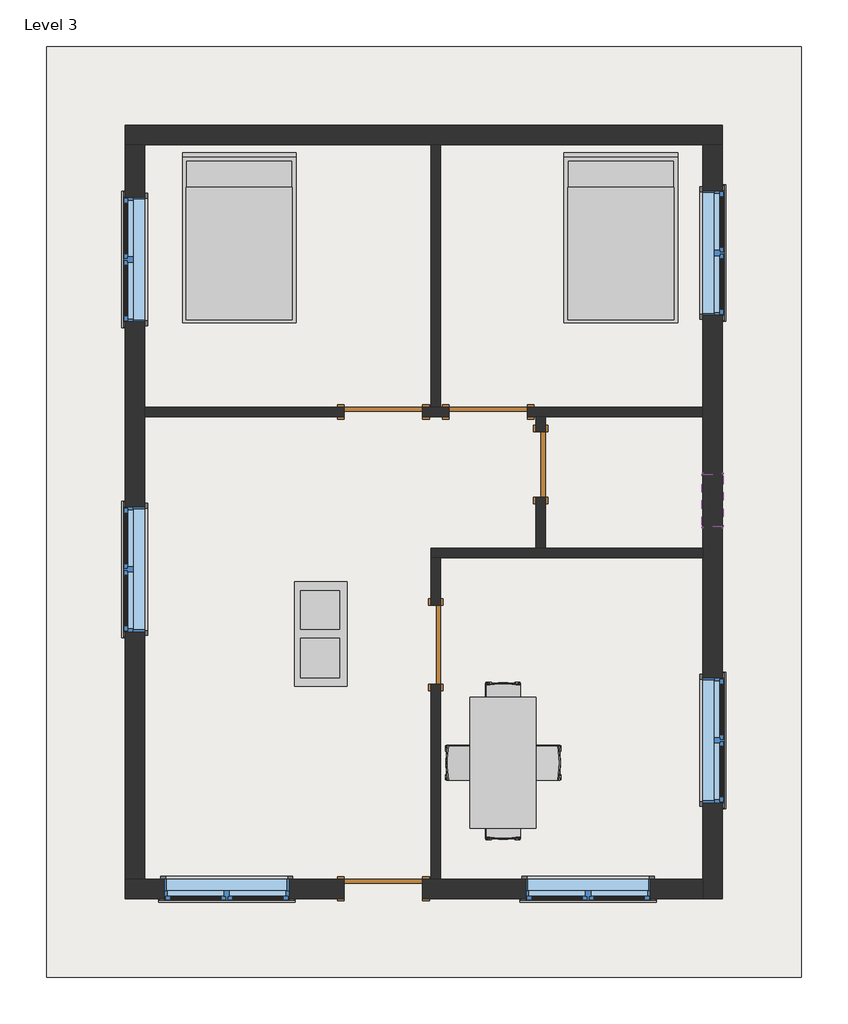
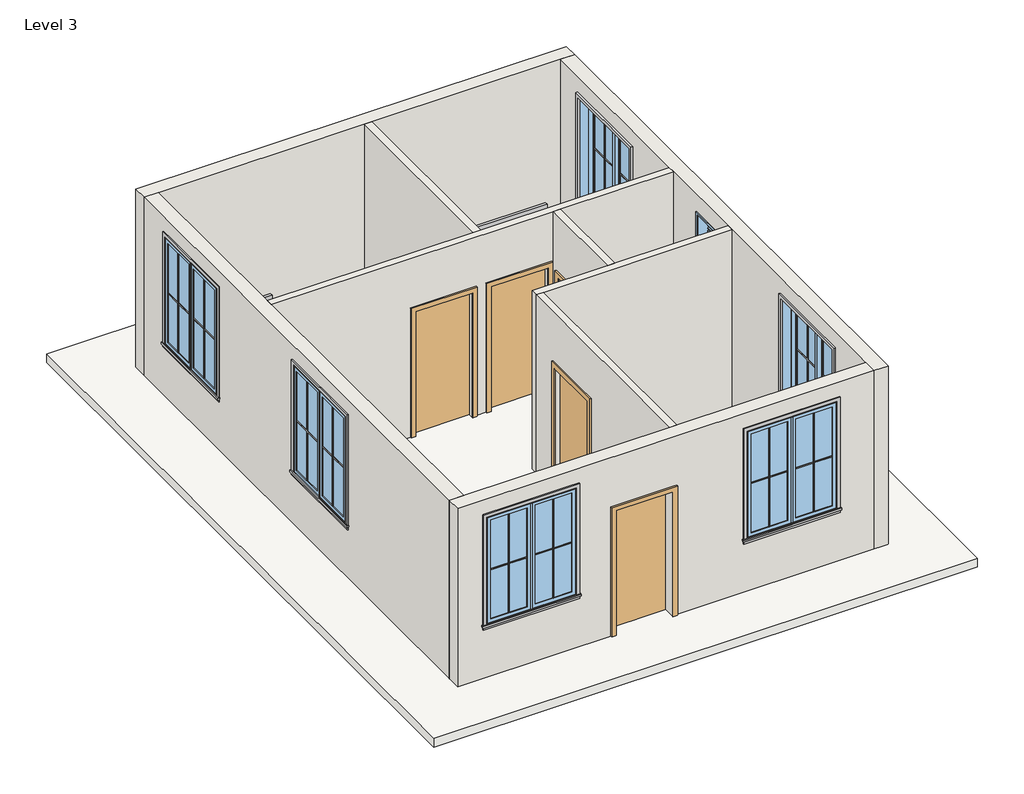
# One storey, incomplete: 25 proxies, 9 walls, 7 windows, 5 doors, 3 furniture elements, 1 roof.
"""IFC4 building model written with IfcOpenShell, lengths in millimetres."""

from ifc_helpers import new_model, si_unit, frame, origin, place, context, project, spatial, polyline, outline, extrude, faceted_brep, transform, mapped, element, save
from components import muntin_pattern_2x2_muntin_pattern_2x2_bff912c5, muntin_pattern_2x2_muntin_pattern_2x2_c2194282, trim_window_exterior_flat_with_sill_e04b3088, trim_window_interior_flat_picture_frame_2a7685fe, coffee_table_with_brass_mullions_11320_coffee_table_with_5962bef7, door_305aa2a5, door_e5f9f3c4, door_0ca8825f, door_f2b275c1, bed_17739_bed_17739_15c61121, dining_table_w_chairs_11374_0cdfc61b, window_9ac97e1a, window_f2d8fef0

model = new_model("IFC4")

# Units and contexts
model_context = context("Model", 3, world=origin())
ifc_project = project(units=[si_unit("LENGTHUNIT", "METRE", prefix="MILLI")], contexts=[model_context])

# Site, building, storey
site = spatial("IfcSite", under=ifc_project)
building = spatial("IfcBuilding", under=site)
storey = spatial("IfcBuildingStorey", under=building, Name="Level 3", Elevation=6248.4)

# Proxies
placement = place(None, origin())
muntin_pattern_2x2_muntin_pattern_2x2_shape = muntin_pattern_2x2_muntin_pattern_2x2_bff912c5(model_context)
element("IfcBuildingElementProxy", 1, Name="Muntin Pattern_2x2 : Muntin Pattern_2x2", ObjectType="Muntin Pattern_2x2 : Muntin Pattern_2x2", at=placement, inside=storey, context=model_context, shape_type="MappedRepresentation", body=[
    mapped(muntin_pattern_2x2_muntin_pattern_2x2_shape, transform((-4718.1437352, -1580.3188735, 7232.65), x_axis=(0.0, 1.0, 0.0), y_axis=(-1.0, 0.0, 0.0), z_axis=(0.0, 0.0, 1.0))),
])
element("IfcBuildingElementProxy", 2, Name="Muntin Pattern_2x2 : Muntin Pattern_2x2", ObjectType="Muntin Pattern_2x2 : Muntin Pattern_2x2", at=placement, inside=storey, context=model_context, shape_type="MappedRepresentation", body=[
    mapped(muntin_pattern_2x2_muntin_pattern_2x2_shape, transform((-3186.2062352, -5039.4813735, 7232.65), x_axis=(-1.0, 0.0, 0.0), y_axis=(0.0, -1.0, 0.0), z_axis=(0.0, 0.0, 1.0))),
])
element("IfcBuildingElementProxy", 3, Name="Muntin Pattern_2x2 : Muntin Pattern_2x2", ObjectType="Muntin Pattern_2x2 : Muntin Pattern_2x2", at=placement, inside=storey, context=model_context, shape_type="MappedRepresentation", body=[
    mapped(muntin_pattern_2x2_muntin_pattern_2x2_shape, transform((1017.4937648, -5039.4813735, 7232.65), x_axis=(-1.0, 0.0, 0.0), y_axis=(0.0, -1.0, 0.0), z_axis=(0.0, 0.0, 1.0))),
])
element("IfcBuildingElementProxy", 4, Name="Muntin Pattern_2x2 : Muntin Pattern_2x2", ObjectType="Muntin Pattern_2x2 : Muntin Pattern_2x2", at=placement, inside=storey, context=model_context, shape_type="MappedRepresentation", body=[
    mapped(muntin_pattern_2x2_muntin_pattern_2x2_shape, transform((2209.7062648, -2847.1438735, 7232.65), x_axis=(0.0, -1.0, 0.0), y_axis=(1.0, 0.0, 0.0), z_axis=(0.0, 0.0, 1.0))),
])
element("IfcBuildingElementProxy", 5, Name="Muntin Pattern_2x2 : Muntin Pattern_2x2", ObjectType="Muntin Pattern_2x2 : Muntin Pattern_2x2", at=placement, inside=storey, context=model_context, shape_type="MappedRepresentation", body=[
    mapped(muntin_pattern_2x2_muntin_pattern_2x2_shape, transform((2209.7062648, 2817.0561265, 7232.65), x_axis=(0.0, -1.0, 0.0), y_axis=(1.0, 0.0, 0.0), z_axis=(0.0, 0.0, 1.0))),
])
element("IfcBuildingElementProxy", 6, Name="Muntin Pattern_2x2 : Muntin Pattern_2x2", ObjectType="Muntin Pattern_2x2 : Muntin Pattern_2x2", at=placement, inside=storey, context=model_context, shape_type="MappedRepresentation", body=[
    mapped(muntin_pattern_2x2_muntin_pattern_2x2_shape, transform((-4718.1437352, 2020.1311265, 7232.65), x_axis=(0.0, 1.0, 0.0), y_axis=(-1.0, 0.0, 0.0), z_axis=(0.0, 0.0, 1.0))),
])
muntin_pattern_2x2_muntin_pattern_2x2_2_shape = muntin_pattern_2x2_muntin_pattern_2x2_c2194282(model_context)
element("IfcBuildingElementProxy", 7, Name="Muntin Pattern_2x2 : Muntin Pattern_2x2", ObjectType="Muntin Pattern_2x2 : Muntin Pattern_2x2", at=placement, inside=storey, context=model_context, shape_type="MappedRepresentation", body=[
    mapped(muntin_pattern_2x2_muntin_pattern_2x2_2_shape, transform((-4718.1437352, -859.5938735, 7232.65), x_axis=(0.0, -1.0, 0.0), y_axis=(1.0, 0.0, 0.0), z_axis=(0.0, 0.0, 1.0))),
])
element("IfcBuildingElementProxy", 8, Name="Muntin Pattern_2x2 : Muntin Pattern_2x2", ObjectType="Muntin Pattern_2x2 : Muntin Pattern_2x2", at=placement, inside=storey, context=model_context, shape_type="MappedRepresentation", body=[
    mapped(muntin_pattern_2x2_muntin_pattern_2x2_2_shape, transform((-3906.9312352, -5039.4813735, 7232.65), x_axis=(1.0, 0.0, 0.0), y_axis=(0.0, 1.0, 0.0), z_axis=(0.0, 0.0, 1.0))),
])
element("IfcBuildingElementProxy", 9, Name="Muntin Pattern_2x2 : Muntin Pattern_2x2", ObjectType="Muntin Pattern_2x2 : Muntin Pattern_2x2", at=placement, inside=storey, context=model_context, shape_type="MappedRepresentation", body=[
    mapped(muntin_pattern_2x2_muntin_pattern_2x2_2_shape, transform((296.7687648, -5039.4813735, 7232.65), x_axis=(1.0, 0.0, 0.0), y_axis=(0.0, 1.0, 0.0), z_axis=(0.0, 0.0, 1.0))),
])
element("IfcBuildingElementProxy", 10, Name="Muntin Pattern_2x2 : Muntin Pattern_2x2", ObjectType="Muntin Pattern_2x2 : Muntin Pattern_2x2", at=placement, inside=storey, context=model_context, shape_type="MappedRepresentation", body=[
    mapped(muntin_pattern_2x2_muntin_pattern_2x2_2_shape, transform((2209.7062648, -3567.8688735, 7232.65), x_axis=(0.0, 1.0, 0.0), y_axis=(-1.0, 0.0, 0.0), z_axis=(0.0, 0.0, 1.0))),
])
element("IfcBuildingElementProxy", 11, Name="Muntin Pattern_2x2 : Muntin Pattern_2x2", ObjectType="Muntin Pattern_2x2 : Muntin Pattern_2x2", at=placement, inside=storey, context=model_context, shape_type="MappedRepresentation", body=[
    mapped(muntin_pattern_2x2_muntin_pattern_2x2_2_shape, transform((2209.7062648, 2096.3311265, 7232.65), x_axis=(0.0, 1.0, 0.0), y_axis=(-1.0, 0.0, 0.0), z_axis=(0.0, 0.0, 1.0))),
])
element("IfcBuildingElementProxy", 12, Name="Muntin Pattern_2x2 : Muntin Pattern_2x2", ObjectType="Muntin Pattern_2x2 : Muntin Pattern_2x2", at=placement, inside=storey, context=model_context, shape_type="MappedRepresentation", body=[
    mapped(muntin_pattern_2x2_muntin_pattern_2x2_2_shape, transform((-4718.1437352, 2740.8561265, 7232.65), x_axis=(0.0, -1.0, 0.0), y_axis=(1.0, 0.0, 0.0), z_axis=(0.0, 0.0, 1.0))),
])
trim_window_exterior_flat_with_sill_shape = trim_window_exterior_flat_with_sill_e04b3088(model_context)
element("IfcBuildingElementProxy", 13, Name="Trim-Window-Exterior-Flat : with Sill", ObjectType="Trim-Window-Exterior-Flat : with Sill", at=placement, inside=storey, context=model_context, shape_type="MappedRepresentation", body=[
    mapped(trim_window_exterior_flat_with_sill_shape, transform((-4727.6687352, -1219.9563735, 8991.6), x_axis=(0.0, -1.0, 0.0), y_axis=(0.0, 0.0, 1.0), z_axis=(-1.0, 0.0, 0.0))),
])
element("IfcBuildingElementProxy", 14, Name="Trim-Window-Exterior-Flat : with Sill", ObjectType="Trim-Window-Exterior-Flat : with Sill", at=placement, inside=storey, context=model_context, shape_type="MappedRepresentation", body=[
    mapped(trim_window_exterior_flat_with_sill_shape, transform((-3546.5687352, -5049.0063735, 8991.6), x_axis=(1.0, 0.0, 0.0), y_axis=(0.0, 0.0, 1.0), z_axis=(0.0, -1.0, 0.0))),
])
element("IfcBuildingElementProxy", 15, Name="Trim-Window-Exterior-Flat : with Sill", ObjectType="Trim-Window-Exterior-Flat : with Sill", at=placement, inside=storey, context=model_context, shape_type="MappedRepresentation", body=[
    mapped(trim_window_exterior_flat_with_sill_shape, transform((657.1312648, -5049.0063735, 8991.6), x_axis=(1.0, 0.0, 0.0), y_axis=(0.0, 0.0, 1.0), z_axis=(0.0, -1.0, 0.0))),
])
element("IfcBuildingElementProxy", 16, Name="Trim-Window-Exterior-Flat : with Sill", ObjectType="Trim-Window-Exterior-Flat : with Sill", at=placement, inside=storey, context=model_context, shape_type="MappedRepresentation", body=[
    mapped(trim_window_exterior_flat_with_sill_shape, transform((2219.2312648, -3207.5063735, 8991.6), x_axis=(0.0, 1.0, 0.0), y_axis=(0.0, 0.0, 1.0), z_axis=(1.0, 0.0, 0.0))),
])
element("IfcBuildingElementProxy", 17, Name="Trim-Window-Exterior-Flat : with Sill", ObjectType="Trim-Window-Exterior-Flat : with Sill", at=placement, inside=storey, context=model_context, shape_type="MappedRepresentation", body=[
    mapped(trim_window_exterior_flat_with_sill_shape, transform((2219.2312648, 2456.6936265, 8991.6), x_axis=(0.0, 1.0, 0.0), y_axis=(0.0, 0.0, 1.0), z_axis=(1.0, 0.0, 0.0))),
])
element("IfcBuildingElementProxy", 18, Name="Trim-Window-Exterior-Flat : with Sill", ObjectType="Trim-Window-Exterior-Flat : with Sill", at=placement, inside=storey, context=model_context, shape_type="MappedRepresentation", body=[
    mapped(trim_window_exterior_flat_with_sill_shape, transform((-4727.6687352, 2380.4936265, 8991.6), x_axis=(0.0, -1.0, 0.0), y_axis=(0.0, 0.0, 1.0), z_axis=(-1.0, 0.0, 0.0))),
])
trim_window_interior_flat_picture_frame_shape = trim_window_interior_flat_picture_frame_2a7685fe(model_context)
element("IfcBuildingElementProxy", 19, Name="Trim-Window-Interior-Flat : Picture Frame", ObjectType="Trim-Window-Interior-Flat : Picture Frame", at=placement, inside=storey, context=model_context, shape_type="MappedRepresentation", body=[
    mapped(trim_window_interior_flat_picture_frame_shape, transform((-4499.0687352, -1219.9563735, 8991.6), x_axis=(0.0, 1.0, 0.0), y_axis=(0.0, 0.0, 1.0), z_axis=(1.0, 0.0, 0.0))),
])
element("IfcBuildingElementProxy", 20, Name="Trim-Window-Interior-Flat : Picture Frame", ObjectType="Trim-Window-Interior-Flat : Picture Frame", at=placement, inside=storey, context=model_context, shape_type="MappedRepresentation", body=[
    mapped(trim_window_interior_flat_picture_frame_shape, transform((-3546.5687352, -4820.4063735, 8991.6), x_axis=(-1.0, 0.0, 0.0), y_axis=(0.0, 0.0, 1.0), z_axis=(0.0, 1.0, 0.0))),
])
element("IfcBuildingElementProxy", 21, Name="Trim-Window-Interior-Flat : Picture Frame", ObjectType="Trim-Window-Interior-Flat : Picture Frame", at=placement, inside=storey, context=model_context, shape_type="MappedRepresentation", body=[
    mapped(trim_window_interior_flat_picture_frame_shape, transform((657.1312648, -4820.4063735, 8991.6), x_axis=(-1.0, 0.0, 0.0), y_axis=(0.0, 0.0, 1.0), z_axis=(0.0, 1.0, 0.0))),
])
element("IfcBuildingElementProxy", 22, Name="Trim-Window-Interior-Flat : Picture Frame", ObjectType="Trim-Window-Interior-Flat : Picture Frame", at=placement, inside=storey, context=model_context, shape_type="MappedRepresentation", body=[
    mapped(trim_window_interior_flat_picture_frame_shape, transform((1990.6312648, -3207.5063735, 8991.6), x_axis=(0.0, -1.0, 0.0), y_axis=(0.0, 0.0, 1.0), z_axis=(-1.0, 0.0, 0.0))),
])
element("IfcBuildingElementProxy", 23, Name="Trim-Window-Interior-Flat : Picture Frame", ObjectType="Trim-Window-Interior-Flat : Picture Frame", at=placement, inside=storey, context=model_context, shape_type="MappedRepresentation", body=[
    mapped(trim_window_interior_flat_picture_frame_shape, transform((1990.6312648, 2456.6936265, 8991.6), x_axis=(0.0, -1.0, 0.0), y_axis=(0.0, 0.0, 1.0), z_axis=(-1.0, 0.0, 0.0))),
])
element("IfcBuildingElementProxy", 24, Name="Trim-Window-Interior-Flat : Picture Frame", ObjectType="Trim-Window-Interior-Flat : Picture Frame", at=placement, inside=storey, context=model_context, shape_type="MappedRepresentation", body=[
    mapped(trim_window_interior_flat_picture_frame_shape, transform((-4499.0687352, 2380.4936265, 8991.6), x_axis=(0.0, 1.0, 0.0), y_axis=(0.0, 0.0, 1.0), z_axis=(1.0, 0.0, 0.0))),
])
coffee_table_with_brass_mullions_11320_coffee_table_with_shape = coffee_table_with_brass_mullions_11320_coffee_table_with_5962bef7(model_context)
element("IfcBuildingElementProxy", 25, Name="coffee_table_with_brass_mullions_11320 : coffee_table_with_brass_mullions_11320", ObjectType="coffee_table_with_brass_mullions_11320 : coffee_table_with_brass_mullions_11320", at=placement, inside=storey, context=model_context, shape_type="MappedRepresentation", body=[
    mapped(coffee_table_with_brass_mullions_11320_coffee_table_with_shape, transform((-2022.5687352, -1334.2563735, 6248.4), x_axis=(0.0, 1.0, 0.0), y_axis=(-1.0, 0.0, 0.0), z_axis=(0.0, 0.0, 1.0))),
])

# Doors
door_shape = door_305aa2a5(model_context)
element("IfcDoor", 26, ObjectType="Single-Flush : 36\" x 84\"", at=placement, inside=storey, context=model_context, shape_type="MappedRepresentation", body=[
    mapped(door_shape, transform((-1114.5187352, -2096.2563735, 6248.4), x_axis=(0.0, 1.0, 0.0), y_axis=(-1.0, 0.0, 0.0), z_axis=(0.0, 0.0, 1.0))),
])
element("IfcDoor", 27, ObjectType="Single-Flush : 36\" x 84\"", at=placement, inside=storey, context=model_context, shape_type="MappedRepresentation", body=[
    mapped(door_shape, transform((-1724.1187352, 608.8436265, 6248.4), x_axis=(-1.0, 0.0, 0.0), y_axis=(0.0, -1.0, 0.0), z_axis=(0.0, 0.0, 1.0))),
])
door_2_shape = door_e5f9f3c4(model_context)
element("IfcDoor", 28, ObjectType="Single-Flush : 36\" x 84\"", at=placement, inside=storey, context=model_context, shape_type="MappedRepresentation", body=[
    mapped(door_2_shape, transform((-504.9187352, 608.8436265, 6248.4), x_axis=(1.0, 0.0, 0.0), y_axis=(0.0, 1.0, 0.0), z_axis=(0.0, 0.0, 1.0))),
])
door_3_shape = door_0ca8825f(model_context)
element("IfcDoor", 29, ObjectType="Single-Flush : 36\" x 84\"", at=placement, inside=storey, context=model_context, shape_type="MappedRepresentation", body=[
    mapped(door_3_shape, transform((-1724.1187352, -4934.7063735, 6248.4), x_axis=(1.0, 0.0, 0.0), y_axis=(0.0, 1.0, 0.0), z_axis=(0.0, 0.0, 1.0))),
])
door_4_shape = door_f2b275c1(model_context)
element("IfcDoor", 30, ObjectType="Single-Flush : DOOR 2'6\"", at=placement, inside=storey, context=model_context, shape_type="MappedRepresentation", body=[
    mapped(door_4_shape, transform((104.6812648, -0.7563735, 6248.4), x_axis=(0.0, 1.0, 0.0), y_axis=(-1.0, 0.0, 0.0), z_axis=(0.0, 0.0, 1.0))),
])

# Furniture
bed_17739_bed_17739_shape = bed_17739_bed_17739_15c61121(model_context)
element("IfcFurniture", 31, ObjectType="Bed_17739 : Bed_17739", at=placement, inside=storey, context=model_context, shape_type="MappedRepresentation", body=[
    mapped(bed_17739_bed_17739_shape, transform((-3400.5187352, 2609.0936265, 6248.4), x_axis=(1.0, 0.0, 0.0), y_axis=(0.0, 1.0, 0.0), z_axis=(0.0, 0.0, 1.0))),
])
element("IfcFurniture", 32, ObjectType="Bed_17739 : Bed_17739", at=placement, inside=storey, context=model_context, shape_type="MappedRepresentation", body=[
    mapped(bed_17739_bed_17739_shape, transform((1038.1312648, 2609.0936265, 6248.4), x_axis=(1.0, 0.0, 0.0), y_axis=(0.0, 1.0, 0.0), z_axis=(0.0, 0.0, 1.0))),
])
dining_table_w_chairs_11374_shape = dining_table_w_chairs_11374_0cdfc61b(model_context)
element("IfcFurniture", 33, ObjectType="Dining_Table_w_Chairs_11374", at=placement, inside=storey, context=model_context, shape_type="MappedRepresentation", body=[
    mapped(dining_table_w_chairs_11374_shape, transform((-238.2576574, -3486.1221401, 6248.4), x_axis=(0.0, 1.0, 0.0), y_axis=(-1.0, 0.0, 0.0), z_axis=(0.0, 0.0, 1.0))),
])

# Roof
element("IfcRoof", 34, ObjectType="ROOF 6\"", at=placement, inside=storey, context=model_context, shape_type="SweptSolid", body=[
    extrude(outline(polyline([(-5642.0687352, 4856.9936265), (3133.6312648, 4856.9936265), (3133.6312648, -5963.4063735), (-5642.0687352, -5963.4063735), (-5642.0687352, 4856.9936265)])), frame((0.0, 0.0, 6096.0), z_axis=(0.0, 0.0, 1.0), x_axis=(1.0, 0.0, 0.0)), (0.0, 0.0, 1.0), 152.4),
])

# Walls
element("IfcWall", 35, ObjectType="WALL 4.5\"", at=placement, inside=storey, context=model_context, shape_type="Brep", body=[
    faceted_brep([(-4499.0687352, 551.6936265, 6248.4), (-2181.3187352, 551.6936265, 6248.4), (-2181.3187352, 551.6936265, 8382.0), (-1266.9187352, 551.6936265, 8382.0), (-1266.9187352, 551.6936265, 6248.4), (-962.1187352, 551.6936265, 6248.4), (-962.1187352, 551.6936265, 8382.0), (-47.7187352, 551.6936265, 8382.0), (-47.7187352, 551.6936265, 6248.4), (47.5312648, 551.6936265, 6248.4), (161.8312648, 551.6936265, 6248.4), (1990.6312648, 551.6936265, 6248.4), (1990.6312648, 551.6936265, 9296.4), (161.8312648, 551.6936265, 9296.4), (47.5312648, 551.6936265, 9296.4), (-4499.0687352, 551.6936265, 9296.4), (-2181.3187352, 665.9936265, 8382.0), (-2181.3187352, 665.9936265, 6248.4), (-4499.0687352, 665.9936265, 6248.4), (-4499.0687352, 665.9936265, 9296.4), (-1171.6687352, 665.9936265, 9296.4), (-1057.3687352, 665.9936265, 9296.4), (1990.6312648, 665.9936265, 9296.4), (1990.6312648, 665.9936265, 6248.4), (-47.7187352, 665.9936265, 6248.4), (-47.7187352, 665.9936265, 8382.0), (-962.1187352, 665.9936265, 8382.0), (-962.1187352, 665.9936265, 6248.4), (-1057.3687352, 665.9936265, 6248.4), (-1171.6687352, 665.9936265, 6248.4), (-1266.9187352, 665.9936265, 6248.4), (-1266.9187352, 665.9936265, 8382.0)], [[[0, 1, 2, 3, 4, 5, 6, 7, 8, 9, 10, 11, 12, 13, 14, 15]], [[16, 17, 18, 19, 20, 21, 22, 23, 24, 25, 26, 27, 28, 29, 30, 31]], [[11, 10, 9, 8, 24, 23]], [[18, 17, 1, 0]], [[30, 29, 28, 27, 5, 4]], [[12, 11, 23, 22]], [[0, 15, 19, 18]], [[25, 24, 8, 7]], [[26, 25, 7, 6]], [[27, 26, 6, 5]], [[2, 1, 17, 16]], [[3, 2, 16, 31]], [[4, 3, 31, 30]], [[15, 14, 13, 12, 22, 21, 20, 19]]]),
])
element("IfcWall", 36, ObjectType="WALL 4.5\"", at=placement, inside=storey, context=model_context, shape_type="SweptSolid", body=[
    extrude(outline(polyline([(-1057.3687352, 3713.9936265), (-1057.3687352, 665.9936265), (-1171.6687352, 665.9936265), (-1171.6687352, 3713.9936265), (-1057.3687352, 3713.9936265)])), frame((0.0, 0.0, 6248.4), z_axis=(0.0, 0.0, 1.0), x_axis=(1.0, 0.0, 0.0)), (0.0, 0.0, 1.0), 3048.0),
])
element("IfcWall", 37, ObjectType="WALL 4.5\"", at=placement, inside=storey, context=model_context, shape_type="Brep", body=[
    faceted_brep([(1990.6312648, -972.3063735, 6248.4), (161.8312648, -972.3063735, 6248.4), (47.5312648, -972.3063735, 6248.4), (-1171.6687352, -972.3063735, 6248.4), (-1171.6687352, -972.3063735, 9296.4), (47.5312648, -972.3063735, 9296.4), (161.8312648, -972.3063735, 9296.4), (1990.6312648, -972.3063735, 9296.4), (1990.6312648, -1086.6063735, 6248.4), (1990.6312648, -1086.6063735, 9296.4), (-1057.3687352, -1086.6063735, 9296.4), (-1171.6687352, -1086.6063735, 9296.4), (-1171.6687352, -1086.6063735, 6248.4), (-1057.3687352, -1086.6063735, 6248.4)], [[[0, 1, 2, 3, 4, 5, 6, 7]], [[8, 9, 10, 11, 12, 13]], [[3, 2, 1, 0, 8, 13, 12]], [[0, 7, 9, 8]], [[4, 3, 12, 11]], [[7, 6, 5, 4, 11, 10, 9]]]),
])
element("IfcWall", 38, ObjectType="WALL 4.5\"", at=placement, inside=storey, context=model_context, shape_type="SweptSolid", body=[
    extrude(outline(polyline([(-1086.6063735, 6248.4), (-1639.0563735, 6248.4), (-1639.0563735, 8382.0), (-2553.4563735, 8382.0), (-2553.4563735, 6248.4), (-4820.4063735, 6248.4), (-4820.4063735, 9296.4), (-1086.6063735, 9296.4), (-1086.6063735, 6248.4)])), frame((-1171.6687352, 0.0, 0.0), z_axis=(1.0, 0.0, 0.0), x_axis=(0.0, 1.0, 0.0)), (0.0, 0.0, 1.0), 114.3),
])
element("IfcWall", 39, ObjectType="WALL 4.5\"", at=placement, inside=storey, context=model_context, shape_type="SweptSolid", body=[
    extrude(outline(polyline([(551.6936265, 6248.4), (380.2436265, 6248.4), (380.2436265, 8280.4), (-381.7563735, 8280.4), (-381.7563735, 6248.4), (-972.3063735, 6248.4), (-972.3063735, 9296.4), (551.6936265, 9296.4), (551.6936265, 6248.4)])), frame((47.5312648, 0.0, 0.0), z_axis=(1.0, 0.0, 0.0), x_axis=(0.0, 1.0, 0.0)), (0.0, 0.0, 1.0), 114.3),
])
element("IfcWall", 40, ObjectType="WALL 9\"", at=placement, inside=storey, context=model_context, shape_type="Brep", body=[
    faceted_brep([(-4727.6687352, 3713.9936265, 6248.4), (-4499.0687352, 3713.9936265, 6248.4), (-1171.6687352, 3713.9936265, 6248.4), (-1057.3687352, 3713.9936265, 6248.4), (1990.6312648, 3713.9936265, 6248.4), (2219.2312648, 3713.9936265, 6248.4), (2219.2312648, 3713.9936265, 9296.4), (1990.6312648, 3713.9936265, 9296.4), (-1057.3687352, 3713.9936265, 9296.4), (-1171.6687352, 3713.9936265, 9296.4), (-4499.0687352, 3713.9936265, 9296.4), (-4727.6687352, 3713.9936265, 9296.4), (-4727.6687352, 3942.5936265, 6248.4), (-4727.6687352, 3942.5936265, 9296.4), (2219.2312648, 3942.5936265, 9296.4), (2219.2312648, 3942.5936265, 6248.4)], [[[0, 1, 2, 3, 4, 5, 6, 7, 8, 9, 10, 11]], [[12, 13, 14, 15]], [[5, 4, 3, 2, 1, 0, 12, 15]], [[6, 5, 15, 14]], [[0, 11, 13, 12]], [[11, 10, 9, 8, 7, 6, 14, 13]]]),
])
element("IfcWall", 41, ObjectType="WALL 9\"", at=placement, inside=storey, context=model_context, shape_type="Brep", body=[
    faceted_brep([(1990.6312648, 3713.9936265, 6248.4), (1990.6312648, 665.9936265, 6248.4), (1990.6312648, 551.6936265, 6248.4), (1990.6312648, -972.3063735, 6248.4), (1990.6312648, -1086.6063735, 6248.4), (1990.6312648, -4820.4063735, 6248.4), (1990.6312648, -5049.0063735, 6248.4), (1990.6312648, -5049.0063735, 9296.4), (1990.6312648, -4820.4063735, 9296.4), (1990.6312648, -1086.6063735, 9296.4), (1990.6312648, -972.3063735, 9296.4), (1990.6312648, 551.6936265, 9296.4), (1990.6312648, 665.9936265, 9296.4), (1990.6312648, 3713.9936265, 9296.4), (1990.6312648, -3931.4063735, 8991.6), (1990.6312648, -3931.4063735, 7162.8), (1990.6312648, -2483.6063735, 7162.8), (1990.6312648, -2483.6063735, 8991.6), (1990.6312648, 1732.7936265, 8991.6), (1990.6312648, 1732.7936265, 7162.8), (1990.6312648, 3180.5936265, 7162.8), (1990.6312648, 3180.5936265, 8991.6), (1990.6312648, -115.0563735, 8991.6), (1990.6312648, -724.6563735, 8991.6), (1990.6312648, -724.6563735, 8382.0), (1990.6312648, -115.0563735, 8382.0), (2219.2312648, 3713.9936265, 6248.4), (2219.2312648, 3713.9936265, 9296.4), (2219.2312648, -5049.0063735, 9296.4), (2219.2312648, -5049.0063735, 6248.4), (2219.2312648, -3931.4063735, 8991.6), (2219.2312648, -2483.6063735, 8991.6), (2219.2312648, -2483.6063735, 7162.8), (2219.2312648, -3931.4063735, 7162.8), (2219.2312648, 1732.7936265, 8991.6), (2219.2312648, 3180.5936265, 8991.6), (2219.2312648, 3180.5936265, 7162.8), (2219.2312648, 1732.7936265, 7162.8), (2219.2312648, -115.0563735, 8991.6), (2219.2312648, -115.0563735, 8382.0), (2219.2312648, -724.6563735, 8382.0), (2219.2312648, -724.6563735, 8991.6)], [[[0, 1, 2, 3, 4, 5, 6, 7, 8, 9, 10, 11, 12, 13], [14, 15, 16, 17], [18, 19, 20, 21], [22, 23, 24, 25]], [[26, 27, 28, 29], [30, 31, 32, 33], [34, 35, 36, 37], [38, 39, 40, 41]], [[6, 5, 4, 3, 2, 1, 0, 26, 29]], [[0, 13, 27, 26]], [[7, 6, 29, 28]], [[15, 14, 30, 33]], [[16, 15, 33, 32]], [[17, 16, 32, 31]], [[14, 17, 31, 30]], [[19, 18, 34, 37]], [[20, 19, 37, 36]], [[21, 20, 36, 35]], [[18, 21, 35, 34]], [[39, 38, 22, 25]], [[40, 39, 25, 24]], [[41, 40, 24, 23]], [[38, 41, 23, 22]], [[13, 12, 11, 10, 9, 8, 7, 28, 27]]]),
])
element("IfcWall", 42, ObjectType="WALL 9\"", at=placement, inside=storey, context=model_context, shape_type="Brep", body=[
    faceted_brep([(1990.6312648, -4820.4063735, 6248.4), (-1057.3687352, -4820.4063735, 6248.4), (-1171.6687352, -4820.4063735, 6248.4), (-1266.9187352, -4820.4063735, 6248.4), (-1266.9187352, -4820.4063735, 8382.0), (-2181.3187352, -4820.4063735, 8382.0), (-2181.3187352, -4820.4063735, 6248.4), (-4499.0687352, -4820.4063735, 6248.4), (-4727.6687352, -4820.4063735, 6248.4), (-4727.6687352, -4820.4063735, 9296.4), (-4499.0687352, -4820.4063735, 9296.4), (-1171.6687352, -4820.4063735, 9296.4), (-1057.3687352, -4820.4063735, 9296.4), (1990.6312648, -4820.4063735, 9296.4), (-4270.4687352, -4820.4063735, 8991.6), (-4270.4687352, -4820.4063735, 7162.8), (-2822.6687352, -4820.4063735, 7162.8), (-2822.6687352, -4820.4063735, 8991.6), (-66.7687352, -4820.4063735, 8991.6), (-66.7687352, -4820.4063735, 7162.8), (1381.0312648, -4820.4063735, 7162.8), (1381.0312648, -4820.4063735, 8991.6), (-1266.9187352, -5049.0063735, 8382.0), (-1266.9187352, -5049.0063735, 6248.4), (1990.6312648, -5049.0063735, 6248.4), (1990.6312648, -5049.0063735, 9296.4), (-4727.6687352, -5049.0063735, 9296.4), (-4727.6687352, -5049.0063735, 6248.4), (-2181.3187352, -5049.0063735, 6248.4), (-2181.3187352, -5049.0063735, 8382.0), (-4270.4687352, -5049.0063735, 8991.6), (-2822.6687352, -5049.0063735, 8991.6), (-2822.6687352, -5049.0063735, 7162.8), (-4270.4687352, -5049.0063735, 7162.8), (-66.7687352, -5049.0063735, 8991.6), (1381.0312648, -5049.0063735, 8991.6), (1381.0312648, -5049.0063735, 7162.8), (-66.7687352, -5049.0063735, 7162.8)], [[[0, 1, 2, 3, 4, 5, 6, 7, 8, 9, 10, 11, 12, 13], [14, 15, 16, 17], [18, 19, 20, 21]], [[22, 23, 24, 25, 26, 27, 28, 29], [30, 31, 32, 33], [34, 35, 36, 37]], [[28, 27, 8, 7, 6]], [[24, 23, 3, 2, 1, 0]], [[0, 13, 25, 24]], [[9, 8, 27, 26]], [[15, 14, 30, 33]], [[16, 15, 33, 32]], [[17, 16, 32, 31]], [[14, 17, 31, 30]], [[19, 18, 34, 37]], [[20, 19, 37, 36]], [[21, 20, 36, 35]], [[18, 21, 35, 34]], [[4, 3, 23, 22]], [[5, 4, 22, 29]], [[6, 5, 29, 28]], [[13, 12, 11, 10, 9, 26, 25]]]),
])
element("IfcWall", 43, ObjectType="WALL 9\"", at=placement, inside=storey, context=model_context, shape_type="Brep", body=[
    faceted_brep([(-4499.0687352, -4820.4063735, 6248.4), (-4499.0687352, 551.6936265, 6248.4), (-4499.0687352, 665.9936265, 6248.4), (-4499.0687352, 3713.9936265, 6248.4), (-4499.0687352, 3713.9936265, 9296.4), (-4499.0687352, 665.9936265, 9296.4), (-4499.0687352, 551.6936265, 9296.4), (-4499.0687352, -4820.4063735, 9296.4), (-4499.0687352, -496.0563735, 8991.6), (-4499.0687352, -496.0563735, 7162.8), (-4499.0687352, -1943.8563735, 7162.8), (-4499.0687352, -1943.8563735, 8991.6), (-4499.0687352, 3104.3936265, 8991.6), (-4499.0687352, 3104.3936265, 7162.8), (-4499.0687352, 1656.5936265, 7162.8), (-4499.0687352, 1656.5936265, 8991.6), (-4727.6687352, -4820.4063735, 6248.4), (-4727.6687352, -4820.4063735, 9296.4), (-4727.6687352, 3713.9936265, 9296.4), (-4727.6687352, 3713.9936265, 6248.4), (-4727.6687352, -496.0563735, 8991.6), (-4727.6687352, -1943.8563735, 8991.6), (-4727.6687352, -1943.8563735, 7162.8), (-4727.6687352, -496.0563735, 7162.8), (-4727.6687352, 3104.3936265, 8991.6), (-4727.6687352, 1656.5936265, 8991.6), (-4727.6687352, 1656.5936265, 7162.8), (-4727.6687352, 3104.3936265, 7162.8)], [[[0, 1, 2, 3, 4, 5, 6, 7], [8, 9, 10, 11], [12, 13, 14, 15]], [[16, 17, 18, 19], [20, 21, 22, 23], [24, 25, 26, 27]], [[3, 2, 1, 0, 16, 19]], [[4, 3, 19, 18]], [[0, 7, 17, 16]], [[9, 8, 20, 23]], [[10, 9, 23, 22]], [[11, 10, 22, 21]], [[8, 11, 21, 20]], [[13, 12, 24, 27]], [[14, 13, 27, 26]], [[15, 14, 26, 25]], [[12, 15, 25, 24]], [[7, 6, 5, 4, 18, 17]]]),
])

# Windows
window_shape = window_9ac97e1a(model_context)
element("IfcWindow", 44, ObjectType="Window-Casement-Double : 57\" x 72\"", at=placement, inside=storey, context=model_context, shape_type="MappedRepresentation", body=[
    mapped(window_shape, transform((-4613.3687352, -1219.9563735, 6248.4), x_axis=(0.0, 1.0, 0.0), y_axis=(-1.0, 0.0, 0.0), z_axis=(0.0, 0.0, 1.0))),
])
element("IfcWindow", 45, ObjectType="Window-Casement-Double : 57\" x 72\"", at=placement, inside=storey, context=model_context, shape_type="MappedRepresentation", body=[
    mapped(window_shape, transform((-3546.5687352, -4934.7063735, 6248.4), x_axis=(-1.0, 0.0, 0.0), y_axis=(0.0, -1.0, 0.0), z_axis=(0.0, 0.0, 1.0))),
])
element("IfcWindow", 46, ObjectType="Window-Casement-Double : 57\" x 72\"", at=placement, inside=storey, context=model_context, shape_type="MappedRepresentation", body=[
    mapped(window_shape, transform((657.1312648, -4934.7063735, 6248.4), x_axis=(-1.0, 0.0, 0.0), y_axis=(0.0, -1.0, 0.0), z_axis=(0.0, 0.0, 1.0))),
])
element("IfcWindow", 47, ObjectType="Window-Casement-Double : 57\" x 72\"", at=placement, inside=storey, context=model_context, shape_type="MappedRepresentation", body=[
    mapped(window_shape, transform((2104.9312648, -3207.5063735, 6248.4), x_axis=(0.0, -1.0, 0.0), y_axis=(1.0, 0.0, 0.0), z_axis=(0.0, 0.0, 1.0))),
])
element("IfcWindow", 48, ObjectType="Window-Casement-Double : 57\" x 72\"", at=placement, inside=storey, context=model_context, shape_type="MappedRepresentation", body=[
    mapped(window_shape, transform((2104.9312648, 2456.6936265, 6248.4), x_axis=(0.0, -1.0, 0.0), y_axis=(1.0, 0.0, 0.0), z_axis=(0.0, 0.0, 1.0))),
])
element("IfcWindow", 49, ObjectType="Window-Casement-Double : 57\" x 72\"", at=placement, inside=storey, context=model_context, shape_type="MappedRepresentation", body=[
    mapped(window_shape, transform((-4613.3687352, 2380.4936265, 6248.4), x_axis=(0.0, 1.0, 0.0), y_axis=(-1.0, 0.0, 0.0), z_axis=(0.0, 0.0, 1.0))),
])
window_2_shape = window_f2d8fef0(model_context)
element("IfcWindow", 50, ObjectType="Window-Louvers : 24\" x 24\"", at=placement, inside=storey, context=model_context, shape_type="MappedRepresentation", body=[
    mapped(window_2_shape, transform((2111.2812648, -419.8563735, 7467.6), x_axis=(0.0, -1.0, 0.0), y_axis=(1.0, 0.0, 0.0), z_axis=(0.0, 0.0, 1.0))),
])

save(model, "model.ifc")

# Revit data of these elements
# Type "Muntin Pattern_2x2 : Muntin Pattern_2x2"
#   Width [instance default] = 4' - 0"
#   Thickness = 0' - 0 1/2"
#   Height [instance default] = 4' - 0"
#   Distance = 0' - 0 3/4"
#   Interior Material [instance default] = none
#   Exterior Material [instance default] = none
#   Default Elevation = 0
# Type "Trim-Window-Exterior-Flat : with Sill"
#   Trim Width = 0' - 2 1/4"
#   Trim Thickness_Picture Frame = 0' - 1 1/4"
#   Trim Thickness_with Sill = 0' - 0 3/4"
#   Sill Thickness = 0' - 1 1/4"
#   Opening Width [instance default] = 2' - 0"
#   Opening Height [instance default] = 3' - 0"
#   Default Elevation = 4' - 0"
#   Sill = yes
#   Picture Frame = no
#   Trim Material [instance default] = none
# Type "Trim-Window-Interior-Flat : Picture Frame"
#   Trim Thickness_Picture Frame = 0' - 1 1/4"
#   Trim Width = 0' - 2 1/4"
#   Trim Thickness_with Sill = 0' - 0 3/4"
#   Sill Thickness = 0' - 1 1/4"
#   Opening Width [instance default] = 2' - 0"
#   Opening Height [instance default] = 3' - 0"
#   Default Elevation = 4' - 0"
#   Sill = no
#   Picture Frame = yes
#   Trim Material [instance default] = none
# Type "coffee_table_with_brass_mullions_11320 : coffee_table_with_brass_mullions_11320"
#   Default Elevation = 0
# Type "Single-Flush : 36\" x 84\""
#   Type Mark = "1"
#   Construction Type Id = "MDOOR"
#   Assembly Code = "C1020"
#   Analytic Construction = "Metal"
#   Thickness = 0' - 2"
#   Heat Transfer Coefficient (U) = 0.651978 BTU/(h·ft²·°F)
#   Height = 7' - 0"
#   Trim Projection Ext = 0' - 1"
#   Trim Projection Int = 0' - 1"
#   Trim Width = 0' - 3"
#   Width = 3' - 0"
#   Define Thermal Properties by = 1
#   Define Thermal Properties by = 1
#   Door Material = Door - Panel
#   Frame Material = Door - Frame
#   Visual Light Transmittance = 0
#   Solar Heat Gain Coefficient = 0
#   Function = (empty or 0)
#   Wall Closure = (empty or 0)
# Type "Single-Flush : DOOR 2'6\""
#   Type Mark = "8"
#   Construction Type Id = "MDOOR"
#   Assembly Code = "C1020"
#   Analytic Construction = "Metal"
#   Thickness = 0' - 2"
#   Heat Transfer Coefficient (U) = 0.651978 BTU/(h·ft²·°F)
#   Height = 6' - 8"
#   Trim Projection Ext = 0' - 1"
#   Trim Projection Int = 0' - 1"
#   Trim Width = 0' - 3"
#   Width = 2' - 6"
#   Define Thermal Properties by = 1
#   Door Material = Door - Panel
#   Frame Material = Door - Frame
#   Visual Light Transmittance = 0
#   Solar Heat Gain Coefficient = 0
#   Function = (empty or 0)
#   Wall Closure = (empty or 0)
# Type "Bed_17739 : Bed_17739"
#   Default Elevation = 0
# Type "Dining_Table_w_Chairs_11374"
#   Default Elevation = 0
#   Assembly Code = ""
# Type "ROOF 6\""
#   Assembly Code = "B1020"
#   Layers, outside or top first: 0' - 6" no material (function 1)
# Type "WALL 4.5\""
#   Assembly Code = "B2010"
#   Layers, outside or top first: 0' - 4 1/2" no material (function 1)
# Type "WALL 9\""
#   Assembly Code = "B2010"
#   Layers, outside or top first: 0' - 9" no material (function 1)
# Type "Window-Casement-Double : 57\" x 72\""
#   Type Mark = "17"
#   Fire Rating = "0.5h"
#   Assembly Code = "B2020100"
#   Analytic Construction = "Double glazing - domestic"
#   Frame Extension [instance default] = 0' - 0 1/4"
#   Window Inset [instance default] = 0' - 0"
#   Wall Thickness [instance default] = 0' - 6"
#   Interior Wall Closure [instance default] = 0' - 2 1/4"
#   Half Width = 2' - 4 1/2"
#   Visual Light Transmittance = 0.81
#   Thermal Resistance (R) = 1.8146 (h·ft²·°F)/BTU
#   Solar Heat Gain Coefficient = 0.76
#   Rough Width = 4' - 9 1/2"
#   Rough Height = 6' - 0 1/2"
#   Height = 6' - 0"
#   Heat Transfer Coefficient (U) = 0.5511 BTU/(h·ft²·°F)
#   Exterior Wall Closure [instance default] = 0' - 1 1/4"
#   Extension Jamb [instance default] = 0' - 2 1/4"
#   Default Sill Height = 3' - 0"
#   Width = 4' - 9"
#   Define Thermal Properties by = 0
#   Muntin Visibility = yes
#   Interior Trim Visibility [instance default] = yes
#   Exterior Trim Visibility [instance default] = yes
#   Extension Jamb Visibility [instance default] = yes
#   Interior Trim Material = Wood - Stained
#   Muntin Pattern = Muntin Pattern_2x2 : Muntin Pattern_2x2
#   Interior Trim = Trim-Window-Interior-Flat : Picture Frame
#   Interior Frame Material = Wood - Stained
#   Glass Panel Material = Glass
#   Exterior Trim Material = Clad - White
#   Exterior Trim = Trim-Window-Exterior-Flat : with Sill
#   Exterior Frame Material = Clad - White
#   Wall Closure = (empty or 0)
# Type "Window-Louvers : 24\" x 24\""
#   Type Mark = "18"
#   Construction Type Id = "GSP4R"
#   Assembly Code = "B20"
#   Analytic Construction = "1/8 in Pilkington single glazing"
#   Visual Light Transmittance = 0.9
#   Thermal Resistance (R) = 1.53941 (h·ft²·°F)/BTU
#   Solar Heat Gain Coefficient = 0.78
#   Max Height = 1' - 11.74264"
#   Height = 2' - 0"
#   Heat Transfer Coefficient (U) = 0.6496 BTU/(h·ft²·°F)
#   Blade Width [instance default] = 1' - 10 1/2"
#   Blade Vertical Thickness = 0' - 0.35355"
#   Blade Thickness = 0' - 0 1/4"
#   Blade Spacing = 0' - 1 1/2"
#   Blade Height = 0' - 1.85355"
#   Blade Depth = 0' - 3"
#   Blade Angle = 45.00°
#   Default Sill Height = 3' - 0"
#   Trim Projection_Exterior = 0' - 0 1/2"
#   Trim Projection_Interior = 0' - 0 1/2"
#   Trim Width_Exterior = 0' - 1 1/2"
#   Trim Width_Interior = 0' - 1 1/2"
#   Width = 2' - 0"
#   Max Blade Count = 12
#   Define Thermal Properties by = 1
#   Blade Count = 12
#   Frame Material = Birch
#   Louver Material = Birch
#   Trim Exterior Material = Birch
#   Trim Interior Material = Birch
#   Wall Closure = (empty or 0)
# Elements 1, 2, 3, 4, 5, 6, 7, 8, 9, 10, 11, 12 (IfcBuildingElementProxy, "Muntin Pattern_2x2 : Muntin Pattern_2x2")
#   Width = 1' - 11 1/8"
#   Height = 5' - 6 1/2"
#   Interior Material = Wood - Stained
#   Exterior Material = Clad - White
#   Phase Created = New Construction
#   Materials on its faces: "Clad - White", "Wood - Stained"
# Elements 13, 14, 15, 16, 17, 18 (IfcBuildingElementProxy, "Trim-Window-Exterior-Flat : with Sill")
#   Opening Width = 4' - 9"
#   Opening Height = 6' - 0"
#   Trim Material = Clad - White
#   Phase Created = New Construction
#   Materials on its faces: "Clad - White"
# Elements 19, 20, 21, 22, 23, 24 (IfcBuildingElementProxy, "Trim-Window-Interior-Flat : Picture Frame")
#   Opening Width = 4' - 9"
#   Opening Height = 6' - 0"
#   Trim Material = Wood - Stained
#   Phase Created = New Construction
#   Materials on its faces: "Wood - Stained"
# Element 25 (IfcBuildingElementProxy, "coffee_table_with_brass_mullions_11320 : coffee_table_with_brass_mullions_11320")
#   Phase Created = New Construction
#   Materials on its faces: "Default Wall", "TABLE", "Glass", "Default"
# Elements 26, 27, 28, 29 (IfcDoor, "Single-Flush : 36\" x 84\"")
#   Phase Created = New Construction
#   Materials on its faces: "Door - Frame", "Door - Panel"
# Element 30 (IfcDoor, "Single-Flush : DOOR 2'6\"")
#   Phase Created = New Construction
#   Materials on its faces: "Door - Frame", "Door - Panel"
# Elements 31, 32 (IfcFurniture, "Bed_17739 : Bed_17739")
#   Phase Created = New Construction
#   Materials on its faces: "legs", "sheets", "bed frame", "Blanket"
# Element 33 (IfcFurniture, "Dining_Table_w_Chairs_11374")
#   Phase Created = New Construction
# Element 34 (IfcRoof, "ROOF 6\"")
#   built-in parameter 1001705 = 20.5 (stored number, unit not read)
#   built-in parameter 1001701 = -0.5 (stored number, unit not read)
#   built-in parameter 1001710 = 33615
#   Phase Created = New Construction
#   Materials on its faces: "Copper", "Default Roof", "Wood - Stained"
# Elements 35, 36, 37, 38, 39 (IfcWall, "WALL 4.5\"")
#   Top Offset = 0' - 0"
#   Base Offset = 0' - 0"
#   Unconnected Height = 10' - 0"
#   wall height = 10' - 0"
#   Phase Created = New Construction
#   Base Constraint = Level 3
#   Materials on its faces: "Default Wall"
# Elements 40, 41, 42, 43 (IfcWall, "WALL 9\"")
#   Top Offset = 0' - 0"
#   Base Offset = 0' - 0"
#   Unconnected Height = 10' - 0"
#   wall height = 10' - 0"
#   Phase Created = New Construction
#   Base Constraint = Level 3
#   Materials on its faces: "Default Wall", "Parking Stripe"
# Element 44 (IfcWindow, "Window-Casement-Double : 57\" x 72\"")
#   Mark = "15"
#   Window Inset = 0' - 0"
#   Interior Wall Closure = 0' - 2 1/4"
#   Frame Extension = 0' - 0 1/4"
#   Exterior Wall Closure = 0' - 1 1/4"
#   Interior Trim Visibility = yes
#   Exterior Trim Visibility = yes
#   Phase Created = New Construction
#   Materials on its faces: "Wood - Stained", "Glass", "Clad - White"
# Element 45 (IfcWindow, "Window-Casement-Double : 57\" x 72\"")
#   Mark = "16"
#   Window Inset = 0' - 0"
#   Interior Wall Closure = 0' - 2 1/4"
#   Frame Extension = 0' - 0 1/4"
#   Exterior Wall Closure = 0' - 1 1/4"
#   Interior Trim Visibility = yes
#   Exterior Trim Visibility = yes
#   Phase Created = New Construction
#   Materials on its faces: "Wood - Stained", "Glass", "Clad - White"
# Element 46 (IfcWindow, "Window-Casement-Double : 57\" x 72\"")
#   Mark = "17"
#   Window Inset = 0' - 0"
#   Interior Wall Closure = 0' - 2 1/4"
#   Frame Extension = 0' - 0 1/4"
#   Exterior Wall Closure = 0' - 1 1/4"
#   Interior Trim Visibility = yes
#   Exterior Trim Visibility = yes
#   Phase Created = New Construction
#   Materials on its faces: "Wood - Stained", "Glass", "Clad - White"
# Element 47 (IfcWindow, "Window-Casement-Double : 57\" x 72\"")
#   Mark = "18"
#   Window Inset = 0' - 0"
#   Interior Wall Closure = 0' - 2 1/4"
#   Frame Extension = 0' - 0 1/4"
#   Exterior Wall Closure = 0' - 1 1/4"
#   Interior Trim Visibility = yes
#   Exterior Trim Visibility = yes
#   Phase Created = New Construction
#   Materials on its faces: "Wood - Stained", "Glass", "Clad - White"
# Element 48 (IfcWindow, "Window-Casement-Double : 57\" x 72\"")
#   Mark = "19"
#   Window Inset = 0' - 0"
#   Interior Wall Closure = 0' - 2 1/4"
#   Frame Extension = 0' - 0 1/4"
#   Exterior Wall Closure = 0' - 1 1/4"
#   Interior Trim Visibility = yes
#   Exterior Trim Visibility = yes
#   Phase Created = New Construction
#   Materials on its faces: "Wood - Stained", "Glass", "Clad - White"
# Element 49 (IfcWindow, "Window-Casement-Double : 57\" x 72\"")
#   Mark = "20"
#   Window Inset = 0' - 0"
#   Interior Wall Closure = 0' - 2 1/4"
#   Frame Extension = 0' - 0 1/4"
#   Exterior Wall Closure = 0' - 1 1/4"
#   Interior Trim Visibility = yes
#   Exterior Trim Visibility = yes
#   Phase Created = New Construction
#   Materials on its faces: "Wood - Stained", "Glass", "Clad - White"
# Element 50 (IfcWindow, "Window-Louvers : 24\" x 24\"")
#   Mark = "21"
#   Blade Width = 1' - 10 1/2"
#   Phase Created = New Construction
#   Materials on its faces: "Birch"
# Materials
#   "Door - Panel": class "Wood", colour RGB 210 159 95, transparency 0, Cost = 0
#   "Door - Frame": colour RGB 118 70 51, transparency 0, Cost = 0
#   "Wood - Stained": class "Wood", colour RGB 224 178 126, transparency 0, Cost = 0
#   "Glass": class "Glass", colour RGB 0 128 192, transparency 0.75, Description = "Soda Lime Glass", Cost = 0
#   "Clad - White": class "Wood", colour RGB 242 242 238, transparency 0, Cost = 0
#   "Birch": class "Wood", colour RGB 224 178 126, transparency 0, Description = "Betula Alleghaniensis", Cost = 0
#   "Default Wall": colour RGB 128 128 128, transparency 0, Cost = 0
#   "TABLE": class "Generic", colour RGB 120 120 120, transparency 0, Cost = 0
#   "Default": colour RGB 127 127 127, transparency 0, Cost = 0
#   "legs": colour RGB 90 73 37, transparency 0, Cost = 0
#   "sheets": colour RGB 200 195 176, transparency 0, Cost = 0
#   "bed frame": colour RGB 90 73 37, transparency 0, Cost = 0
#   "Blanket": class "System", colour RGB 59 0 1, transparency 0, Cost = 0
#   "Copper": class "Metal", colour RGB 0 0 0, transparency 0, Description = "Copper, matte finish", Cost = 0
#   "Default Roof": colour RGB 88 101 114, transparency 0, Cost = 0
#   "Parking Stripe": class "Paint", colour RGB 250 250 91, transparency 0, Cost = 0
